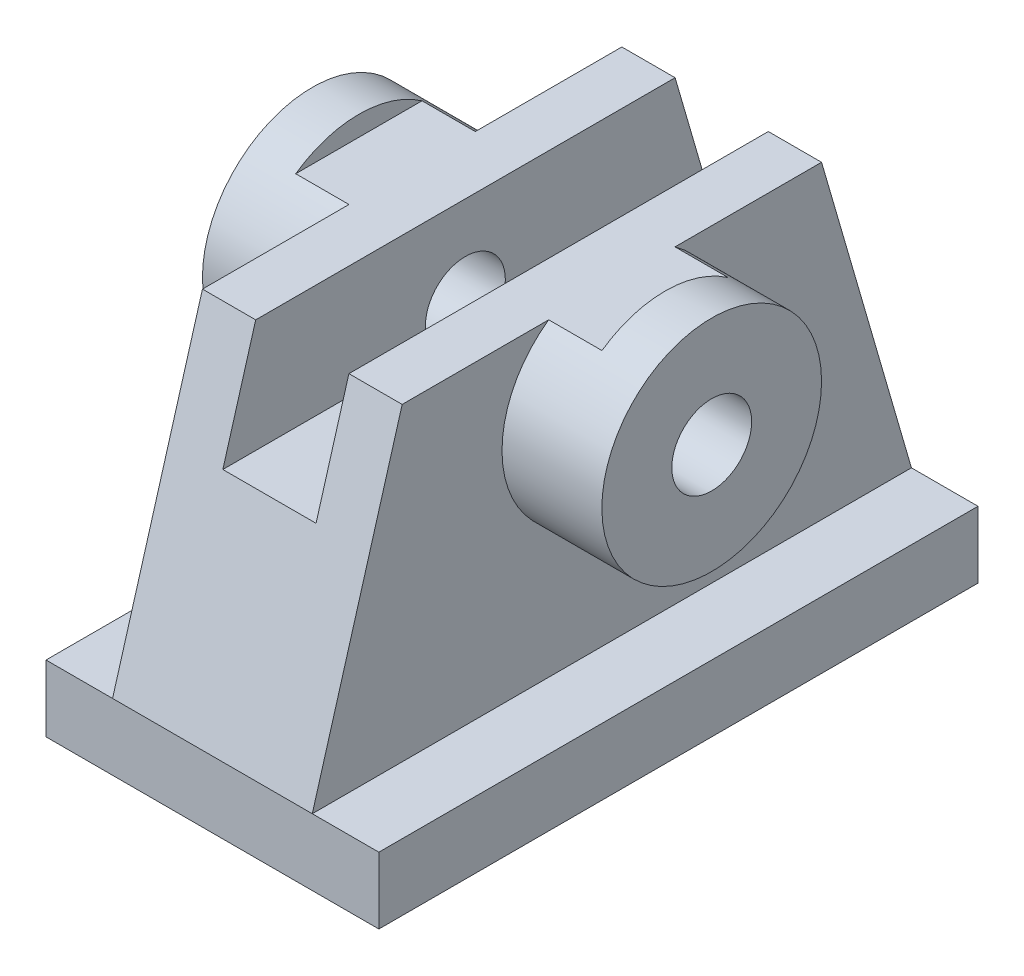
ISO-10303-21;
HEADER;
FILE_DESCRIPTION(('STEP AP214'),'2;1');
FILE_NAME('part.step','',(''),(''),'','','');
FILE_SCHEMA(('AUTOMOTIVE_DESIGN { 1 0 10303 214 1 1 1 1 }'));
ENDSEC;
DATA;
#1=APPLICATION_CONTEXT('core data for automotive mechanical design processes');
#2=APPLICATION_PROTOCOL_DEFINITION('international standard','automotive_design',2000,#1);
#3=PRODUCT_CONTEXT('',#1,'mechanical');
#4=PRODUCT('Part','Part','',(#3));
#5=PRODUCT_RELATED_PRODUCT_CATEGORY('part','',(#4));
#6=PRODUCT_DEFINITION_FORMATION('','',#4);
#7=PRODUCT_DEFINITION_CONTEXT('part definition',#1,'design');
#8=PRODUCT_DEFINITION('design','',#6,#7);
#9=PRODUCT_DEFINITION_SHAPE('','',#8);
#10=(LENGTH_UNIT() NAMED_UNIT(*) SI_UNIT(.MILLI.,.METRE.));
#11=(NAMED_UNIT(*) PLANE_ANGLE_UNIT() SI_UNIT($,.RADIAN.));
#12=(NAMED_UNIT(*) SI_UNIT($,.STERADIAN.) SOLID_ANGLE_UNIT());
#13=UNCERTAINTY_MEASURE_WITH_UNIT(LENGTH_MEASURE(1.E-05),#10,'distance_accuracy_value','');
#14=(GEOMETRIC_REPRESENTATION_CONTEXT(3) GLOBAL_UNCERTAINTY_ASSIGNED_CONTEXT((#13)) GLOBAL_UNIT_ASSIGNED_CONTEXT((#10,
#11,#12)) REPRESENTATION_CONTEXT('',''));
#15=CARTESIAN_POINT('',(0.,0.,0.));
#16=DIRECTION('',(0.,0.,1.));
#17=DIRECTION('',(1.,0.,0.));
#18=AXIS2_PLACEMENT_3D('',#15,#16,#17);
#19=CARTESIAN_POINT('',(-23.,56.5,-65.));
#20=DIRECTION('',(0.,-1.,0.));
#21=DIRECTION('',(1.,0.,0.));
#22=AXIS2_PLACEMENT_3D('',#19,#20,#21);
#23=PLANE('',#22);
#24=DIRECTION('',(0.,0.,1.));
#25=VECTOR('',#24,1.);
#26=CARTESIAN_POINT('',(-7.,56.5,-45.));
#27=LINE('',#26,#25);
#28=CARTESIAN_POINT('',(-6.99999999999999,56.5,-31.5));
#29=VERTEX_POINT('',#28);
#30=CARTESIAN_POINT('',(-6.99999999999999,56.5,31.5));
#31=VERTEX_POINT('',#30);
#32=EDGE_CURVE('E238',#29,#31,#27,.T.);
#33=ORIENTED_EDGE('',*,*,#32,.F.);
#34=DIRECTION('',(1.,0.,0.));
#35=VECTOR('',#34,1.);
#36=CARTESIAN_POINT('',(-65.,56.5,-31.5));
#37=LINE('',#36,#35);
#38=CARTESIAN_POINT('',(-15.,56.5,-31.5));
#39=VERTEX_POINT('',#38);
#40=EDGE_CURVE('E196',#39,#29,#37,.T.);
#41=ORIENTED_EDGE('',*,*,#40,.F.);
#42=DIRECTION('',(0.,0.,-1.));
#43=VECTOR('',#42,1.);
#44=CARTESIAN_POINT('',(-15.,56.5,-45.));
#45=LINE('',#44,#43);
#46=CARTESIAN_POINT('',(-15.,56.5,-9.48683298050512));
#47=VERTEX_POINT('',#46);
#48=EDGE_CURVE('E239',#47,#39,#45,.T.);
#49=ORIENTED_EDGE('',*,*,#48,.F.);
#50=DIRECTION('',(-1.,0.,0.));
#51=VECTOR('',#50,1.);
#52=CARTESIAN_POINT('',(30.,56.5,-9.48683298050511));
#53=LINE('',#52,#51);
#54=CARTESIAN_POINT('',(-23.,56.5,-9.48683298050511));
#55=VERTEX_POINT('',#54);
#56=EDGE_CURVE('E243',#55,#47,#53,.F.);
#57=ORIENTED_EDGE('',*,*,#56,.F.);
#58=DIRECTION('',(0.,0.,1.));
#59=VECTOR('',#58,1.);
#60=CARTESIAN_POINT('',(-23.,56.5,-65.));
#61=LINE('',#60,#59);
#62=CARTESIAN_POINT('',(-23.,56.5,9.48683298050514));
#63=VERTEX_POINT('',#62);
#64=EDGE_CURVE('E229',#55,#63,#61,.T.);
#65=ORIENTED_EDGE('',*,*,#64,.T.);
#66=DIRECTION('',(-1.,0.,0.));
#67=VECTOR('',#66,1.);
#68=CARTESIAN_POINT('',(30.,56.5,9.48683298050514));
#69=LINE('',#68,#67);
#70=CARTESIAN_POINT('',(-15.,56.5,9.48683298050515));
#71=VERTEX_POINT('',#70);
#72=EDGE_CURVE('E246',#71,#63,#69,.T.);
#73=ORIENTED_EDGE('',*,*,#72,.F.);
#74=CARTESIAN_POINT('',(-15.,56.5,31.5));
#75=VERTEX_POINT('',#74);
#76=EDGE_CURVE('E244',#75,#71,#45,.T.);
#77=ORIENTED_EDGE('',*,*,#76,.F.);
#78=DIRECTION('',(1.,0.,0.));
#79=VECTOR('',#78,1.);
#80=CARTESIAN_POINT('',(-65.,56.5,31.5));
#81=LINE('',#80,#79);
#82=EDGE_CURVE('E11',#75,#31,#81,.T.);
#83=ORIENTED_EDGE('',*,*,#82,.T.);
#84=EDGE_LOOP('',(#33,#41,#49,#57,#65,#73,#77,#83));
#85=FACE_BOUND('',#84,.T.);
#86=ADVANCED_FACE('F39',(#85),#23,.F.);
#87=CARTESIAN_POINT('',(-25.,10.,45.));
#88=DIRECTION('',(0.,0.,-1.));
#89=DIRECTION('',(-1.,0.,0.));
#90=AXIS2_PLACEMENT_3D('',#87,#88,#89);
#91=PLANE('',#90);
#92=DIRECTION('',(1.,0.,0.));
#93=VECTOR('',#92,1.);
#94=CARTESIAN_POINT('',(-65.,10.,45.));
#95=LINE('',#94,#93);
#96=CARTESIAN_POINT('',(-15.,10.,45.));
#97=VERTEX_POINT('',#96);
#98=CARTESIAN_POINT('',(15.,10.,45.));
#99=VERTEX_POINT('',#98);
#100=EDGE_CURVE('E194',#97,#99,#95,.T.);
#101=ORIENTED_EDGE('',*,*,#100,.F.);
#102=DIRECTION('',(1.,0.,0.));
#103=VECTOR('',#102,1.);
#104=CARTESIAN_POINT('',(-25.,10.,45.));
#105=LINE('',#104,#103);
#106=CARTESIAN_POINT('',(-25.,10.,45.));
#107=VERTEX_POINT('',#106);
#108=EDGE_CURVE('E292',#107,#97,#105,.T.);
#109=ORIENTED_EDGE('',*,*,#108,.F.);
#110=DIRECTION('',(0.,-1.,0.));
#111=VECTOR('',#110,1.);
#112=CARTESIAN_POINT('',(-25.,10.,45.));
#113=LINE('',#112,#111);
#114=CARTESIAN_POINT('',(-25.,0.,45.));
#115=VERTEX_POINT('',#114);
#116=EDGE_CURVE('E302',#107,#115,#113,.T.);
#117=ORIENTED_EDGE('',*,*,#116,.T.);
#118=DIRECTION('',(1.,0.,0.));
#119=VECTOR('',#118,1.);
#120=CARTESIAN_POINT('',(-25.,0.,45.));
#121=LINE('',#120,#119);
#122=CARTESIAN_POINT('',(25.,0.,45.));
#123=VERTEX_POINT('',#122);
#124=EDGE_CURVE('E281',#115,#123,#121,.T.);
#125=ORIENTED_EDGE('',*,*,#124,.T.);
#126=DIRECTION('',(0.,-1.,0.));
#127=VECTOR('',#126,1.);
#128=CARTESIAN_POINT('',(25.,10.,45.));
#129=LINE('',#128,#127);
#130=CARTESIAN_POINT('',(25.,10.,45.));
#131=VERTEX_POINT('',#130);
#132=EDGE_CURVE('E294',#131,#123,#129,.T.);
#133=ORIENTED_EDGE('',*,*,#132,.F.);
#134=EDGE_CURVE('E289',#99,#131,#105,.T.);
#135=ORIENTED_EDGE('',*,*,#134,.F.);
#136=EDGE_LOOP('',(#101,#109,#117,#125,#133,#135));
#137=FACE_BOUND('',#136,.T.);
#138=ADVANCED_FACE('F348',(#137),#91,.F.);
#139=DIRECTION('',(0.,0.,-1.));
#140=VECTOR('',#139,1.);
#141=CARTESIAN_POINT('',(7.,56.5,-45.));
#142=LINE('',#141,#140);
#143=CARTESIAN_POINT('',(7.00000000000001,56.5,31.5));
#144=VERTEX_POINT('',#143);
#145=CARTESIAN_POINT('',(7.00000000000001,56.5,-31.5));
#146=VERTEX_POINT('',#145);
#147=EDGE_CURVE('E234',#144,#146,#142,.T.);
#148=ORIENTED_EDGE('',*,*,#147,.F.);
#149=CARTESIAN_POINT('',(15.,56.5,31.5));
#150=VERTEX_POINT('',#149);
#151=EDGE_CURVE('E48',#144,#150,#81,.T.);
#152=ORIENTED_EDGE('',*,*,#151,.T.);
#153=DIRECTION('',(0.,0.,1.));
#154=VECTOR('',#153,1.);
#155=CARTESIAN_POINT('',(15.,56.5,-45.));
#156=LINE('',#155,#154);
#157=CARTESIAN_POINT('',(15.,56.5,9.48683298050514));
#158=VERTEX_POINT('',#157);
#159=EDGE_CURVE('E237',#158,#150,#156,.T.);
#160=ORIENTED_EDGE('',*,*,#159,.F.);
#161=DIRECTION('',(-1.,0.,0.));
#162=VECTOR('',#161,1.);
#163=CARTESIAN_POINT('',(30.,56.5,9.48683298050514));
#164=LINE('',#163,#162);
#165=CARTESIAN_POINT('',(23.,56.5,9.48683298050514));
#166=VERTEX_POINT('',#165);
#167=EDGE_CURVE('E316',#166,#158,#164,.T.);
#168=ORIENTED_EDGE('',*,*,#167,.F.);
#169=DIRECTION('',(0.,0.,1.));
#170=VECTOR('',#169,1.);
#171=CARTESIAN_POINT('',(23.,56.5,-65.));
#172=LINE('',#171,#170);
#173=CARTESIAN_POINT('',(23.,56.5,-9.48683298050511));
#174=VERTEX_POINT('',#173);
#175=EDGE_CURVE('E230',#174,#166,#172,.T.);
#176=ORIENTED_EDGE('',*,*,#175,.F.);
#177=DIRECTION('',(-1.,0.,0.));
#178=VECTOR('',#177,1.);
#179=CARTESIAN_POINT('',(30.,56.5,-9.48683298050511));
#180=LINE('',#179,#178);
#181=CARTESIAN_POINT('',(15.,56.5,-9.48683298050511));
#182=VERTEX_POINT('',#181);
#183=EDGE_CURVE('E269',#182,#174,#180,.F.);
#184=ORIENTED_EDGE('',*,*,#183,.F.);
#185=CARTESIAN_POINT('',(15.,56.5,-31.5));
#186=VERTEX_POINT('',#185);
#187=EDGE_CURVE('E233',#186,#182,#156,.T.);
#188=ORIENTED_EDGE('',*,*,#187,.F.);
#189=EDGE_CURVE('E203',#146,#186,#37,.T.);
#190=ORIENTED_EDGE('',*,*,#189,.F.);
#191=EDGE_LOOP('',(#148,#152,#160,#168,#176,#184,#188,#190));
#192=FACE_BOUND('',#191,.T.);
#193=ADVANCED_FACE('F335',(#192),#23,.F.);
#194=CARTESIAN_POINT('',(7.,39.5,-45.));
#195=DIRECTION('',(0.,-1.,0.));
#196=DIRECTION('',(0.,0.,-1.));
#197=AXIS2_PLACEMENT_3D('',#194,#195,#196);
#198=PLANE('',#197);
#199=DIRECTION('',(0.,0.,1.));
#200=VECTOR('',#199,1.);
#201=CARTESIAN_POINT('',(-7.,39.5,-45.));
#202=LINE('',#201,#200);
#203=CARTESIAN_POINT('',(-6.99999999999999,39.5,4.8733971724045));
#204=VERTEX_POINT('',#203);
#205=CARTESIAN_POINT('',(-7.,39.5,36.4354838709677));
#206=VERTEX_POINT('',#205);
#207=EDGE_CURVE('E57',#204,#206,#202,.T.);
#208=ORIENTED_EDGE('',*,*,#207,.T.);
#209=DIRECTION('',(1.,0.,0.));
#210=VECTOR('',#209,1.);
#211=CARTESIAN_POINT('',(7.,39.5,36.4354838709677));
#212=LINE('',#211,#210);
#213=CARTESIAN_POINT('',(7.,39.5,36.4354838709677));
#214=VERTEX_POINT('',#213);
#215=EDGE_CURVE('E61',#206,#214,#212,.T.);
#216=ORIENTED_EDGE('',*,*,#215,.T.);
#217=DIRECTION('',(0.,0.,1.));
#218=VECTOR('',#217,1.);
#219=CARTESIAN_POINT('',(7.,39.5,-45.));
#220=LINE('',#219,#218);
#221=CARTESIAN_POINT('',(7.,39.5,4.87339717240451));
#222=VERTEX_POINT('',#221);
#223=EDGE_CURVE('E178',#222,#214,#220,.T.);
#224=ORIENTED_EDGE('',*,*,#223,.F.);
#225=DIRECTION('',(-1.,0.,0.));
#226=VECTOR('',#225,1.);
#227=CARTESIAN_POINT('',(30.,39.5,4.8733971724045));
#228=LINE('',#227,#226);
#229=EDGE_CURVE('E186',#222,#204,#228,.T.);
#230=ORIENTED_EDGE('',*,*,#229,.T.);
#231=EDGE_LOOP('',(#208,#216,#224,#230));
#232=FACE_BOUND('',#231,.T.);
#233=ADVANCED_FACE('F345',(#232),#198,.F.);
#234=CARTESIAN_POINT('',(7.,39.5,-36.4354838709677));
#235=VERTEX_POINT('',#234);
#236=CARTESIAN_POINT('',(7.,39.5,-4.87339717240447));
#237=VERTEX_POINT('',#236);
#238=EDGE_CURVE('E271',#235,#237,#220,.T.);
#239=ORIENTED_EDGE('',*,*,#238,.F.);
#240=DIRECTION('',(-1.,0.,0.));
#241=VECTOR('',#240,1.);
#242=CARTESIAN_POINT('',(7.,39.5,-36.4354838709677));
#243=LINE('',#242,#241);
#244=CARTESIAN_POINT('',(-7.,39.5,-36.4354838709677));
#245=VERTEX_POINT('',#244);
#246=EDGE_CURVE('E171',#235,#245,#243,.T.);
#247=ORIENTED_EDGE('',*,*,#246,.T.);
#248=CARTESIAN_POINT('',(-6.99999999999999,39.5,-4.87339717240448));
#249=VERTEX_POINT('',#248);
#250=EDGE_CURVE('E169',#245,#249,#202,.T.);
#251=ORIENTED_EDGE('',*,*,#250,.T.);
#252=DIRECTION('',(-1.,0.,0.));
#253=VECTOR('',#252,1.);
#254=CARTESIAN_POINT('',(30.,39.5,-4.87339717240448));
#255=LINE('',#254,#253);
#256=EDGE_CURVE('E174',#249,#237,#255,.F.);
#257=ORIENTED_EDGE('',*,*,#256,.T.);
#258=EDGE_LOOP('',(#239,#247,#251,#257));
#259=FACE_BOUND('',#258,.T.);
#260=ADVANCED_FACE('F168',(#259),#198,.F.);
#261=CARTESIAN_POINT('',(0.,10.,0.));
#262=DIRECTION('',(0.,1.,0.));
#263=DIRECTION('',(0.,0.,1.));
#264=AXIS2_PLACEMENT_3D('',#261,#262,#263);
#265=PLANE('',#264);
#266=DIRECTION('',(0.,0.,-1.));
#267=VECTOR('',#266,1.);
#268=CARTESIAN_POINT('',(15.,10.,-45.));
#269=LINE('',#268,#267);
#270=CARTESIAN_POINT('',(15.,10.,-45.));
#271=VERTEX_POINT('',#270);
#272=EDGE_CURVE('E275',#99,#271,#269,.T.);
#273=ORIENTED_EDGE('',*,*,#272,.F.);
#274=ORIENTED_EDGE('',*,*,#134,.T.);
#275=DIRECTION('',(0.,0.,-1.));
#276=VECTOR('',#275,1.);
#277=CARTESIAN_POINT('',(25.,10.,-45.));
#278=LINE('',#277,#276);
#279=CARTESIAN_POINT('',(25.,10.,-45.));
#280=VERTEX_POINT('',#279);
#281=EDGE_CURVE('E278',#131,#280,#278,.T.);
#282=ORIENTED_EDGE('',*,*,#281,.T.);
#283=DIRECTION('',(-1.,0.,0.));
#284=VECTOR('',#283,1.);
#285=CARTESIAN_POINT('',(-25.,10.,-45.));
#286=LINE('',#285,#284);
#287=EDGE_CURVE('E283',#280,#271,#286,.T.);
#288=ORIENTED_EDGE('',*,*,#287,.T.);
#289=EDGE_LOOP('',(#273,#274,#282,#288));
#290=FACE_BOUND('',#289,.T.);
#291=ADVANCED_FACE('F349',(#290),#265,.T.);
#292=CARTESIAN_POINT('',(25.,10.,-45.));
#293=DIRECTION('',(-1.,0.,0.));
#294=DIRECTION('',(0.,0.,1.));
#295=AXIS2_PLACEMENT_3D('',#292,#293,#294);
#296=PLANE('',#295);
#297=DIRECTION('',(0.,0.,-1.));
#298=VECTOR('',#297,1.);
#299=CARTESIAN_POINT('',(25.,0.,-45.));
#300=LINE('',#299,#298);
#301=CARTESIAN_POINT('',(25.,0.,-45.));
#302=VERTEX_POINT('',#301);
#303=EDGE_CURVE('E276',#123,#302,#300,.T.);
#304=ORIENTED_EDGE('',*,*,#303,.T.);
#305=DIRECTION('',(0.,-1.,0.));
#306=VECTOR('',#305,1.);
#307=CARTESIAN_POINT('',(25.,10.,-45.));
#308=LINE('',#307,#306);
#309=EDGE_CURVE('E270',#280,#302,#308,.T.);
#310=ORIENTED_EDGE('',*,*,#309,.F.);
#311=ORIENTED_EDGE('',*,*,#281,.F.);
#312=ORIENTED_EDGE('',*,*,#132,.T.);
#313=EDGE_LOOP('',(#304,#310,#311,#312));
#314=FACE_BOUND('',#313,.T.);
#315=ADVANCED_FACE('F41',(#314),#296,.F.);
#316=CARTESIAN_POINT('',(-25.,10.,-45.));
#317=DIRECTION('',(0.,0.,1.));
#318=DIRECTION('',(1.,0.,0.));
#319=AXIS2_PLACEMENT_3D('',#316,#317,#318);
#320=PLANE('',#319);
#321=CARTESIAN_POINT('',(-15.,10.,-45.));
#322=VERTEX_POINT('',#321);
#323=CARTESIAN_POINT('',(-25.,10.,-45.));
#324=VERTEX_POINT('',#323);
#325=EDGE_CURVE('E285',#322,#324,#286,.T.);
#326=ORIENTED_EDGE('',*,*,#325,.F.);
#327=DIRECTION('',(1.,0.,0.));
#328=VECTOR('',#327,1.);
#329=CARTESIAN_POINT('',(-65.,10.,-45.));
#330=LINE('',#329,#328);
#331=EDGE_CURVE('E191',#322,#271,#330,.T.);
#332=ORIENTED_EDGE('',*,*,#331,.T.);
#333=ORIENTED_EDGE('',*,*,#287,.F.);
#334=ORIENTED_EDGE('',*,*,#309,.T.);
#335=DIRECTION('',(-1.,0.,0.));
#336=VECTOR('',#335,1.);
#337=CARTESIAN_POINT('',(-25.,0.,-45.));
#338=LINE('',#337,#336);
#339=CARTESIAN_POINT('',(-25.,0.,-45.));
#340=VERTEX_POINT('',#339);
#341=EDGE_CURVE('E299',#302,#340,#338,.T.);
#342=ORIENTED_EDGE('',*,*,#341,.T.);
#343=DIRECTION('',(0.,-1.,0.));
#344=VECTOR('',#343,1.);
#345=CARTESIAN_POINT('',(-25.,10.,-45.));
#346=LINE('',#345,#344);
#347=EDGE_CURVE('E307',#324,#340,#346,.T.);
#348=ORIENTED_EDGE('',*,*,#347,.F.);
#349=EDGE_LOOP('',(#326,#332,#333,#334,#342,#348));
#350=FACE_BOUND('',#349,.T.);
#351=ADVANCED_FACE('F410',(#350),#320,.F.);
#352=CARTESIAN_POINT('',(-25.,10.,-45.));
#353=DIRECTION('',(1.,0.,0.));
#354=DIRECTION('',(0.,0.,-1.));
#355=AXIS2_PLACEMENT_3D('',#352,#353,#354);
#356=PLANE('',#355);
#357=DIRECTION('',(0.,0.,1.));
#358=VECTOR('',#357,1.);
#359=CARTESIAN_POINT('',(-25.,0.,-45.));
#360=LINE('',#359,#358);
#361=EDGE_CURVE('E296',#340,#115,#360,.T.);
#362=ORIENTED_EDGE('',*,*,#361,.T.);
#363=ORIENTED_EDGE('',*,*,#116,.F.);
#364=DIRECTION('',(0.,0.,1.));
#365=VECTOR('',#364,1.);
#366=CARTESIAN_POINT('',(-25.,10.,-45.));
#367=LINE('',#366,#365);
#368=EDGE_CURVE('E286',#324,#107,#367,.T.);
#369=ORIENTED_EDGE('',*,*,#368,.F.);
#370=ORIENTED_EDGE('',*,*,#347,.T.);
#371=EDGE_LOOP('',(#362,#363,#369,#370));
#372=FACE_BOUND('',#371,.T.);
#373=ADVANCED_FACE('F405',(#372),#356,.F.);
#374=DIRECTION('',(0.,0.,1.));
#375=VECTOR('',#374,1.);
#376=CARTESIAN_POINT('',(-15.,10.,-45.));
#377=LINE('',#376,#375);
#378=EDGE_CURVE('E277',#322,#97,#377,.T.);
#379=ORIENTED_EDGE('',*,*,#378,.F.);
#380=ORIENTED_EDGE('',*,*,#325,.T.);
#381=ORIENTED_EDGE('',*,*,#368,.T.);
#382=ORIENTED_EDGE('',*,*,#108,.T.);
#383=EDGE_LOOP('',(#379,#380,#381,#382));
#384=FACE_BOUND('',#383,.T.);
#385=ADVANCED_FACE('F397',(#384),#265,.T.);
#386=CARTESIAN_POINT('',(0.,0.,0.));
#387=DIRECTION('',(0.,1.,0.));
#388=DIRECTION('',(0.,0.,1.));
#389=AXIS2_PLACEMENT_3D('',#386,#387,#388);
#390=PLANE('',#389);
#391=ORIENTED_EDGE('',*,*,#303,.F.);
#392=ORIENTED_EDGE('',*,*,#124,.F.);
#393=ORIENTED_EDGE('',*,*,#361,.F.);
#394=ORIENTED_EDGE('',*,*,#341,.F.);
#395=EDGE_LOOP('',(#391,#392,#393,#394));
#396=FACE_BOUND('',#395,.T.);
#397=ADVANCED_FACE('F396',(#396),#390,.F.);
#398=CARTESIAN_POINT('',(15.,66.5,-45.));
#399=DIRECTION('',(-1.,0.,0.));
#400=DIRECTION('',(0.,0.,1.));
#401=AXIS2_PLACEMENT_3D('',#398,#399,#400);
#402=PLANE('',#401);
#403=ORIENTED_EDGE('',*,*,#159,.T.);
#404=DIRECTION('',(0.,-0.960346226753624,0.278810194863955));
#405=VECTOR('',#404,1.);
#406=CARTESIAN_POINT('',(15.,86.2058541266794,22.8757197696737));
#407=LINE('',#406,#405);
#408=EDGE_CURVE('E221',#150,#99,#407,.T.);
#409=ORIENTED_EDGE('',*,*,#408,.T.);
#410=ORIENTED_EDGE('',*,*,#272,.T.);
#411=DIRECTION('',(0.,0.960346226753624,0.278810194863956));
#412=VECTOR('',#411,1.);
#413=CARTESIAN_POINT('',(15.,62.1079654510557,-29.8718809980806));
#414=LINE('',#413,#412);
#415=EDGE_CURVE('E215',#271,#186,#414,.T.);
#416=ORIENTED_EDGE('',*,*,#415,.T.);
#417=ORIENTED_EDGE('',*,*,#187,.T.);
#418=CARTESIAN_POINT('',(15.,43.,0.));
#419=DIRECTION('',(-1.,0.,0.));
#420=DIRECTION('',(0.,0.,1.));
#421=AXIS2_PLACEMENT_3D('',#418,#419,#420);
#422=CIRCLE('',#421,16.5);
#423=EDGE_CURVE('E266',#158,#182,#422,.F.);
#424=ORIENTED_EDGE('',*,*,#423,.F.);
#425=EDGE_LOOP('',(#403,#409,#410,#416,#417,#424));
#426=FACE_BOUND('',#425,.T.);
#427=ADVANCED_FACE('F328',(#426),#402,.F.);
#428=CARTESIAN_POINT('',(-15.,66.5,-45.));
#429=DIRECTION('',(1.,0.,0.));
#430=DIRECTION('',(0.,0.,-1.));
#431=AXIS2_PLACEMENT_3D('',#428,#429,#430);
#432=PLANE('',#431);
#433=ORIENTED_EDGE('',*,*,#378,.T.);
#434=DIRECTION('',(0.,0.960346226753624,-0.278810194863955));
#435=VECTOR('',#434,1.);
#436=CARTESIAN_POINT('',(-15.,86.2058541266794,22.8757197696737));
#437=LINE('',#436,#435);
#438=EDGE_CURVE('E222',#97,#75,#437,.T.);
#439=ORIENTED_EDGE('',*,*,#438,.T.);
#440=ORIENTED_EDGE('',*,*,#76,.T.);
#441=CARTESIAN_POINT('',(-15.,43.,0.));
#442=DIRECTION('',(1.,0.,0.));
#443=DIRECTION('',(0.,0.,-1.));
#444=AXIS2_PLACEMENT_3D('',#441,#442,#443);
#445=CIRCLE('',#444,16.5);
#446=EDGE_CURVE('E263',#47,#71,#445,.F.);
#447=ORIENTED_EDGE('',*,*,#446,.F.);
#448=ORIENTED_EDGE('',*,*,#48,.T.);
#449=DIRECTION('',(0.,-0.960346226753624,-0.278810194863956));
#450=VECTOR('',#449,1.);
#451=CARTESIAN_POINT('',(-15.,62.1079654510557,-29.8718809980806));
#452=LINE('',#451,#450);
#453=EDGE_CURVE('E207',#39,#322,#452,.T.);
#454=ORIENTED_EDGE('',*,*,#453,.T.);
#455=EDGE_LOOP('',(#433,#439,#440,#447,#448,#454));
#456=FACE_BOUND('',#455,.T.);
#457=ADVANCED_FACE('F386',(#456),#432,.F.);
#458=CARTESIAN_POINT('',(-7.,39.5,-45.));
#459=DIRECTION('',(-1.,0.,0.));
#460=DIRECTION('',(0.,0.,1.));
#461=AXIS2_PLACEMENT_3D('',#458,#459,#460);
#462=PLANE('',#461);
#463=ORIENTED_EDGE('',*,*,#32,.T.);
#464=DIRECTION('',(0.,-0.960346226753624,0.278810194863955));
#465=VECTOR('',#464,1.);
#466=CARTESIAN_POINT('',(-7.,61.3047024952015,30.1050863723609));
#467=LINE('',#466,#465);
#468=EDGE_CURVE('E214',#31,#206,#467,.T.);
#469=ORIENTED_EDGE('',*,*,#468,.T.);
#470=ORIENTED_EDGE('',*,*,#207,.F.);
#471=CARTESIAN_POINT('',(-6.99999999999999,43.,0.));
#472=DIRECTION('',(-1.,0.,0.));
#473=DIRECTION('',(0.,0.,1.));
#474=AXIS2_PLACEMENT_3D('',#471,#472,#473);
#475=CIRCLE('',#474,6.);
#476=EDGE_CURVE('E177',#204,#249,#475,.T.);
#477=ORIENTED_EDGE('',*,*,#476,.T.);
#478=ORIENTED_EDGE('',*,*,#250,.F.);
#479=DIRECTION('',(0.,0.960346226753624,0.278810194863956));
#480=VECTOR('',#479,1.);
#481=CARTESIAN_POINT('',(-7.,37.2068138195777,-37.1012476007678));
#482=LINE('',#481,#480);
#483=EDGE_CURVE('E210',#245,#29,#482,.T.);
#484=ORIENTED_EDGE('',*,*,#483,.T.);
#485=EDGE_LOOP('',(#463,#469,#470,#477,#478,#484));
#486=FACE_BOUND('',#485,.T.);
#487=ADVANCED_FACE('F182',(#486),#462,.F.);
#488=CARTESIAN_POINT('',(7.,39.5,-45.));
#489=DIRECTION('',(1.,0.,0.));
#490=DIRECTION('',(0.,0.,-1.));
#491=AXIS2_PLACEMENT_3D('',#488,#489,#490);
#492=PLANE('',#491);
#493=ORIENTED_EDGE('',*,*,#147,.T.);
#494=DIRECTION('',(0.,-0.960346226753624,-0.278810194863956));
#495=VECTOR('',#494,1.);
#496=CARTESIAN_POINT('',(7.,37.2068138195777,-37.1012476007678));
#497=LINE('',#496,#495);
#498=EDGE_CURVE('E197',#146,#235,#497,.T.);
#499=ORIENTED_EDGE('',*,*,#498,.T.);
#500=ORIENTED_EDGE('',*,*,#238,.T.);
#501=CARTESIAN_POINT('',(7.00000000000001,43.,0.));
#502=DIRECTION('',(1.,0.,0.));
#503=DIRECTION('',(0.,1.,0.));
#504=AXIS2_PLACEMENT_3D('',#501,#502,#503);
#505=CIRCLE('',#504,6.);
#506=EDGE_CURVE('E190',#237,#222,#505,.T.);
#507=ORIENTED_EDGE('',*,*,#506,.T.);
#508=ORIENTED_EDGE('',*,*,#223,.T.);
#509=DIRECTION('',(0.,0.960346226753624,-0.278810194863955));
#510=VECTOR('',#509,1.);
#511=CARTESIAN_POINT('',(7.,61.3047024952015,30.1050863723609));
#512=LINE('',#511,#510);
#513=EDGE_CURVE('E217',#214,#144,#512,.T.);
#514=ORIENTED_EDGE('',*,*,#513,.T.);
#515=EDGE_LOOP('',(#493,#499,#500,#507,#508,#514));
#516=FACE_BOUND('',#515,.T.);
#517=ADVANCED_FACE('F338',(#516),#492,.F.);
#518=CARTESIAN_POINT('',(30.,43.,0.));
#519=DIRECTION('',(-1.,0.,0.));
#520=DIRECTION('',(0.,0.,1.));
#521=AXIS2_PLACEMENT_3D('',#518,#519,#520);
#522=CYLINDRICAL_SURFACE('',#521,16.5);
#523=CARTESIAN_POINT('',(-30.,43.,0.));
#524=DIRECTION('',(1.,0.,0.));
#525=DIRECTION('',(0.,0.,-1.));
#526=AXIS2_PLACEMENT_3D('',#523,#524,#525);
#527=CIRCLE('',#526,16.5);
#528=CARTESIAN_POINT('',(-30.,43.,-16.5));
#529=VERTEX_POINT('',#528);
#530=EDGE_CURVE('E254',#529,#529,#527,.T.);
#531=ORIENTED_EDGE('',*,*,#530,.T.);
#532=EDGE_LOOP('',(#531));
#533=FACE_BOUND('',#532,.T.);
#534=ORIENTED_EDGE('',*,*,#446,.T.);
#535=ORIENTED_EDGE('',*,*,#72,.T.);
#536=CARTESIAN_POINT('',(-23.,43.,0.));
#537=DIRECTION('',(-1.,0.,0.));
#538=DIRECTION('',(0.,0.,1.));
#539=AXIS2_PLACEMENT_3D('',#536,#537,#538);
#540=CIRCLE('',#539,16.5);
#541=EDGE_CURVE('E43',#63,#55,#540,.T.);
#542=ORIENTED_EDGE('',*,*,#541,.T.);
#543=ORIENTED_EDGE('',*,*,#56,.T.);
#544=EDGE_LOOP('',(#534,#535,#542,#543));
#545=FACE_BOUND('',#544,.T.);
#546=ADVANCED_FACE('F377',(#533,#545),#522,.T.);
#547=CARTESIAN_POINT('',(-30.,43.,0.));
#548=DIRECTION('',(1.,0.,0.));
#549=DIRECTION('',(0.,0.,-1.));
#550=AXIS2_PLACEMENT_3D('',#547,#548,#549);
#551=PLANE('',#550);
#552=ORIENTED_EDGE('',*,*,#530,.F.);
#553=EDGE_LOOP('',(#552));
#554=FACE_BOUND('',#553,.T.);
#555=CARTESIAN_POINT('',(-30.,43.,0.));
#556=DIRECTION('',(1.,0.,0.));
#557=DIRECTION('',(0.,0.,-1.));
#558=AXIS2_PLACEMENT_3D('',#555,#556,#557);
#559=CIRCLE('',#558,6.);
#560=CARTESIAN_POINT('',(-30.,43.,-5.99999999999999));
#561=VERTEX_POINT('',#560);
#562=EDGE_CURVE('E253',#561,#561,#559,.T.);
#563=ORIENTED_EDGE('',*,*,#562,.T.);
#564=EDGE_LOOP('',(#563));
#565=FACE_BOUND('',#564,.T.);
#566=ADVANCED_FACE('F376',(#554,#565),#551,.F.);
#567=CARTESIAN_POINT('',(30.,43.,0.));
#568=DIRECTION('',(1.,0.,0.));
#569=DIRECTION('',(0.,0.,-1.));
#570=AXIS2_PLACEMENT_3D('',#567,#568,#569);
#571=CIRCLE('',#570,16.5);
#572=CARTESIAN_POINT('',(30.,43.,-16.5));
#573=VERTEX_POINT('',#572);
#574=EDGE_CURVE('E256',#573,#573,#571,.T.);
#575=ORIENTED_EDGE('',*,*,#574,.F.);
#576=EDGE_LOOP('',(#575));
#577=FACE_BOUND('',#576,.T.);
#578=CARTESIAN_POINT('',(23.,43.,0.));
#579=DIRECTION('',(1.,0.,0.));
#580=DIRECTION('',(0.,0.,-1.));
#581=AXIS2_PLACEMENT_3D('',#578,#579,#580);
#582=CIRCLE('',#581,16.5);
#583=EDGE_CURVE('E314',#174,#166,#582,.T.);
#584=ORIENTED_EDGE('',*,*,#583,.T.);
#585=ORIENTED_EDGE('',*,*,#167,.T.);
#586=ORIENTED_EDGE('',*,*,#423,.T.);
#587=ORIENTED_EDGE('',*,*,#183,.T.);
#588=EDGE_LOOP('',(#584,#585,#586,#587));
#589=FACE_BOUND('',#588,.T.);
#590=ADVANCED_FACE('F331',(#577,#589),#522,.T.);
#591=CARTESIAN_POINT('',(30.,43.,0.));
#592=DIRECTION('',(-1.,0.,0.));
#593=DIRECTION('',(0.,0.,1.));
#594=AXIS2_PLACEMENT_3D('',#591,#592,#593);
#595=CYLINDRICAL_SURFACE('',#594,6.);
#596=ORIENTED_EDGE('',*,*,#506,.F.);
#597=ORIENTED_EDGE('',*,*,#256,.F.);
#598=ORIENTED_EDGE('',*,*,#476,.F.);
#599=ORIENTED_EDGE('',*,*,#229,.F.);
#600=EDGE_LOOP('',(#596,#597,#598,#599));
#601=FACE_BOUND('',#600,.T.);
#602=CARTESIAN_POINT('',(30.,43.,0.));
#603=DIRECTION('',(1.,0.,0.));
#604=DIRECTION('',(0.,0.,-1.));
#605=AXIS2_PLACEMENT_3D('',#602,#603,#604);
#606=CIRCLE('',#605,6.);
#607=CARTESIAN_POINT('',(30.,43.,-5.99999999999999));
#608=VERTEX_POINT('',#607);
#609=EDGE_CURVE('E252',#608,#608,#606,.T.);
#610=ORIENTED_EDGE('',*,*,#609,.T.);
#611=EDGE_LOOP('',(#610));
#612=FACE_BOUND('',#611,.T.);
#613=ORIENTED_EDGE('',*,*,#562,.F.);
#614=EDGE_LOOP('',(#613));
#615=FACE_BOUND('',#614,.T.);
#616=ADVANCED_FACE('F183',(#601,#612,#615),#595,.F.);
#617=CARTESIAN_POINT('',(30.,43.,0.));
#618=DIRECTION('',(1.,0.,0.));
#619=DIRECTION('',(0.,0.,-1.));
#620=AXIS2_PLACEMENT_3D('',#617,#618,#619);
#621=PLANE('',#620);
#622=ORIENTED_EDGE('',*,*,#574,.T.);
#623=EDGE_LOOP('',(#622));
#624=FACE_BOUND('',#623,.T.);
#625=ORIENTED_EDGE('',*,*,#609,.F.);
#626=EDGE_LOOP('',(#625));
#627=FACE_BOUND('',#626,.T.);
#628=ADVANCED_FACE('F369',(#624,#627),#621,.T.);
#629=CARTESIAN_POINT('',(-23.,66.5,-65.));
#630=DIRECTION('',(-1.,0.,0.));
#631=DIRECTION('',(0.,0.,1.));
#632=AXIS2_PLACEMENT_3D('',#629,#630,#631);
#633=PLANE('',#632);
#634=ORIENTED_EDGE('',*,*,#64,.F.);
#635=ORIENTED_EDGE('',*,*,#541,.F.);
#636=EDGE_LOOP('',(#634,#635));
#637=FACE_BOUND('',#636,.T.);
#638=ADVANCED_FACE('F368',(#637),#633,.F.);
#639=CARTESIAN_POINT('',(23.,66.5,-65.));
#640=DIRECTION('',(1.,0.,0.));
#641=DIRECTION('',(0.,0.,-1.));
#642=AXIS2_PLACEMENT_3D('',#639,#640,#641);
#643=PLANE('',#642);
#644=ORIENTED_EDGE('',*,*,#175,.T.);
#645=ORIENTED_EDGE('',*,*,#583,.F.);
#646=EDGE_LOOP('',(#644,#645));
#647=FACE_BOUND('',#646,.T.);
#648=ADVANCED_FACE('F365',(#647),#643,.F.);
#649=CARTESIAN_POINT('',(-65.,56.5,-31.5));
#650=DIRECTION('',(0.,-0.278810194863956,0.960346226753624));
#651=DIRECTION('',(0.,-0.960346226753624,-0.278810194863956));
#652=AXIS2_PLACEMENT_3D('',#649,#650,#651);
#653=PLANE('',#652);
#654=ORIENTED_EDGE('',*,*,#331,.F.);
#655=ORIENTED_EDGE('',*,*,#453,.F.);
#656=ORIENTED_EDGE('',*,*,#40,.T.);
#657=ORIENTED_EDGE('',*,*,#483,.F.);
#658=ORIENTED_EDGE('',*,*,#246,.F.);
#659=ORIENTED_EDGE('',*,*,#498,.F.);
#660=ORIENTED_EDGE('',*,*,#189,.T.);
#661=ORIENTED_EDGE('',*,*,#415,.F.);
#662=EDGE_LOOP('',(#654,#655,#656,#657,#658,#659,#660,#661));
#663=FACE_BOUND('',#662,.T.);
#664=ADVANCED_FACE('F322',(#663),#653,.F.);
#665=CARTESIAN_POINT('',(-65.,56.5,31.5));
#666=DIRECTION('',(0.,-0.278810194863955,-0.960346226753624));
#667=DIRECTION('',(0.,0.960346226753624,-0.278810194863955));
#668=AXIS2_PLACEMENT_3D('',#665,#666,#667);
#669=PLANE('',#668);
#670=ORIENTED_EDGE('',*,*,#151,.F.);
#671=ORIENTED_EDGE('',*,*,#513,.F.);
#672=ORIENTED_EDGE('',*,*,#215,.F.);
#673=ORIENTED_EDGE('',*,*,#468,.F.);
#674=ORIENTED_EDGE('',*,*,#82,.F.);
#675=ORIENTED_EDGE('',*,*,#438,.F.);
#676=ORIENTED_EDGE('',*,*,#100,.T.);
#677=ORIENTED_EDGE('',*,*,#408,.F.);
#678=EDGE_LOOP('',(#670,#671,#672,#673,#674,#675,#676,#677));
#679=FACE_BOUND('',#678,.T.);
#680=ADVANCED_FACE('F339',(#679),#669,.F.);
#681=CLOSED_SHELL('',(#86,#138,#193,#233,#260,#291,#315,#351,#373,#385,#397,#427,#457,#487,#517,
#546,#566,#590,#616,#628,#638,#648,#664,#680));
#682=MANIFOLD_SOLID_BREP('B2',#681);
#683=ADVANCED_BREP_SHAPE_REPRESENTATION('',(#18,#682),#14);
#684=SHAPE_DEFINITION_REPRESENTATION(#9,#683);
ENDSEC;
END-ISO-10303-21;
